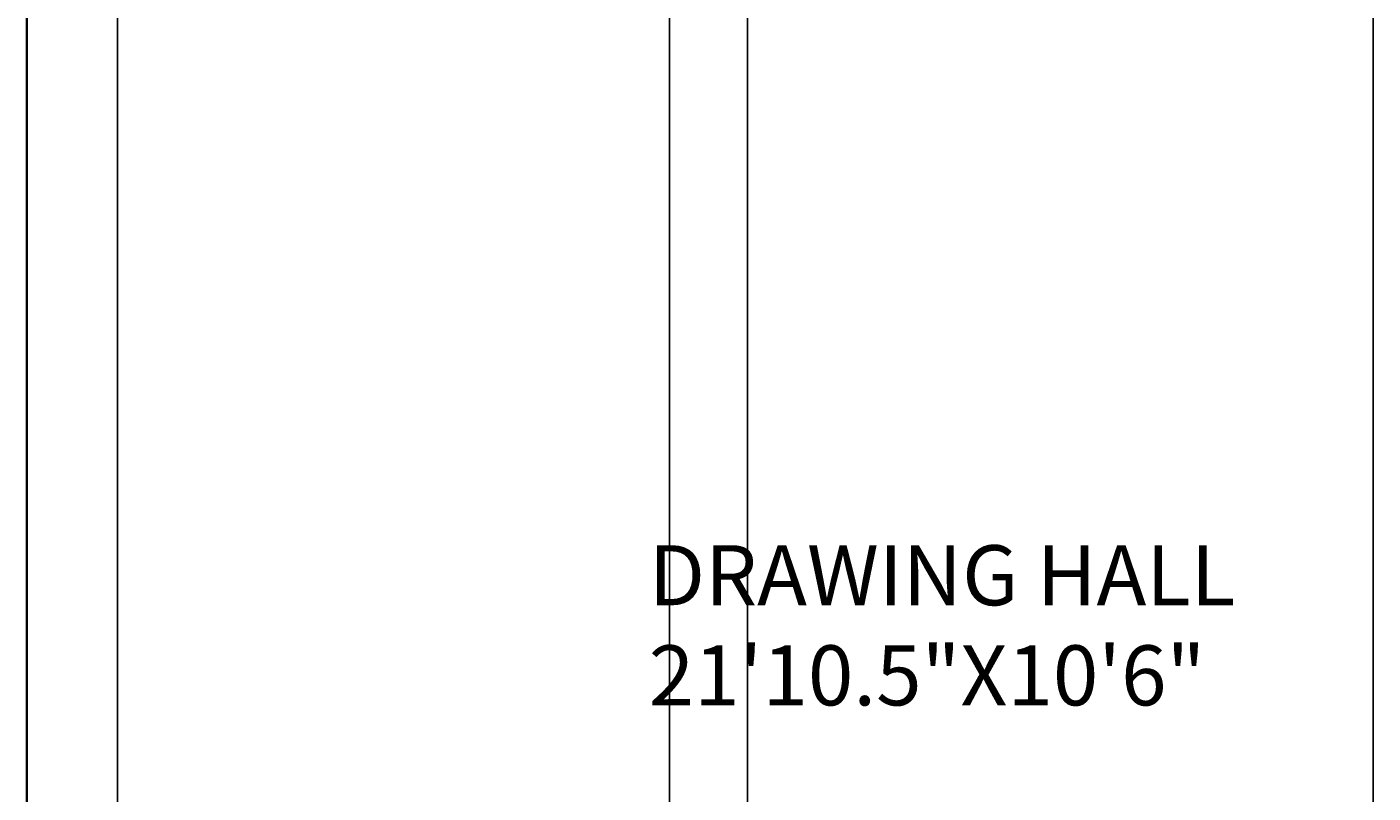
# Model space of a CAD drawing. Units: inches. Extents: x 1088 to 1703, y 668 to 1875.
# Tile 11 of 45: x 1175 to 1309, y 1496 to 1572. Entities that reach past the tile are written whole.
import ezdxf

# ---------------------------------------------------------------- set-up
doc = ezdxf.new("R2010")
doc.units = ezdxf.units.IN
for name, color, linetype, lineweight in [('A-ANNO-DIMS', 2, 'Continuous', 18), ('A-AREA-IDEN', 7, 'Continuous', 18), ('A-WALL', 7, 'Continuous', 35)]:
    doc.layers.add(name, color=color, linetype=linetype, lineweight=lineweight)
doc.styles.get("Standard").update_dxf_attribs({"font": 'arial.ttf'})
doc.dimstyles.get("Standard").update_dxf_attribs({"dimtxt": 0.18, "dimasz": 0.18, "dimexe": 0.18, "dimexo": 0.0625, "dimgap": 0.09, "dimtad": 0, "dimtih": 1, "dimtoh": 1, "dimdec": 4, "dimzin": 0, "dimdsep": 46, "dimtxsty": 'Standard', "dimcen": 0.09, "dimadec": 0, "dimazin": 0, "dimtfac": 1, "dimtdec": 4, "dimtofl": 0, "dimtmove": 0, "dimatfit": 3, "dimfxl": 1, "dimtolj": 1, "dimtzin": 0, "dimarcsym": 0})

# ---------------------------------------------------------------- blocks, each defined once
blk = doc.blocks.new('*D35')
at = {"layer": 'A-ANNO-DIMS', "color": 0, "lineweight": -2, "transparency": 16777216}
for p, q in [((1183.89, 1448.1), (1183.89, 1857.79)), ((1184.07, 1857.61), (1211.07, 1857.61)), ((1238.86, 1857.61), (1211.86, 1857.61)), ((1239.04, 1448.1), (1239.04, 1857.79))]:
    blk.add_line(p, q, dxfattribs=at)
at = {"layer": 'A-ANNO-DIMS', "color": 0, "transparency": 16777216}
for points in [[(1184.07, 1857.64), (1184.07, 1857.58), (1183.89, 1857.61)], [(1238.86, 1857.64), (1238.86, 1857.58), (1239.04, 1857.61)]]:
    blk.add_solid(points, dxfattribs=at)
at = {"layer": 'Defpoints', "color": 0, "transparency": 16777216}
for p in [(1239.04, 1857.61), (1183.89, 1448.04), (1239.04, 1448.04)]:
    blk.add_point(p, dxfattribs=at)
at = {"layer": 'A-ANNO-DIMS', "color": 0, "transparency": 16777216, "insert": (1211.47, 1857.61), "char_height": 0.18, "attachment_point": 5}
blk.add_mtext('\\A1;55.15', dxfattribs=at)
blk = doc.blocks.new('*D36')
at = {"layer": 'A-ANNO-DIMS', "color": 0, "lineweight": -2, "transparency": 16777216}
for p, q in [((1246.85, 1448.35), (1246.85, 1857.79)), ((1247.03, 1857.61), (1277.78, 1857.61)), ((1309.17, 1857.61), (1278.43, 1857.61)), ((1309.35, 1448.35), (1309.35, 1857.79))]:
    blk.add_line(p, q, dxfattribs=at)
at = {"layer": 'A-ANNO-DIMS', "color": 0, "transparency": 16777216}
for points in [[(1247.03, 1857.64), (1247.03, 1857.58), (1246.85, 1857.61)], [(1309.17, 1857.64), (1309.17, 1857.58), (1309.35, 1857.61)]]:
    blk.add_solid(points, dxfattribs=at)
at = {"layer": 'Defpoints', "color": 0, "transparency": 16777216}
for p in [(1309.35, 1857.61), (1246.85, 1448.29), (1309.35, 1448.29)]:
    blk.add_point(p, dxfattribs=at)
at = {"layer": 'A-ANNO-DIMS', "color": 0, "transparency": 16777216, "insert": (1278.1, 1857.61), "char_height": 0.18, "attachment_point": 5}
blk.add_mtext('\\A1;62.5', dxfattribs=at)

msp = doc.modelspace()

# ---------------------------------------------------------------- linework, layer by layer
at = {"layer": 'A-WALL'}
msp.add_line((1174.845, 1644.558), (1174.845, 1419.144), dxfattribs=at)

# ---------------------------------------------------------------- texts
at = {"layer": 'A-AREA-IDEN', "insert": (1236.976, 1520.44), "char_height": 6, "attachment_point": 1}
msp.add_mtext_dynamic_manual_height_columns('DRAWING HALL\\P21\'10.5"X10\'6"', width=114.28689, gutter_width=12.5, heights=[0], dxfattribs=at)

# ---------------------------------------------------------------- dimensions: what is measured, and where the dimension line sits
at = {"layer": 'A-ANNO-DIMS'}
for base, p1, p2, override, picture, middle in [((1239.039, 1857.608), (1183.893, 1448.04), (1239.039, 1448.04), {"dimdec": 2, "dimlfac": 1, "dimrnd": 0, "dimzin": 0, "dimdsep": 46, "dimlunit": 2}, '*D35', (1211.466, 1857.608)), ((1309.352, 1857.608), (1246.852, 1448.287), (1309.352, 1448.287), {"dimdec": 1, "dimlfac": 1, "dimrnd": 0, "dimzin": 0, "dimdsep": 46, "dimlunit": 2}, '*D36', (1278.102, 1857.608))]:
    dim = msp.add_linear_dim(base=base, p1=p1, p2=p2, dimstyle='Standard', override=override, dxfattribs=at)
    dim.commit()
    dim.dimension.update_dxf_attribs({"geometry": picture, "text_midpoint": middle})

doc.saveas('drawing.dxf')
